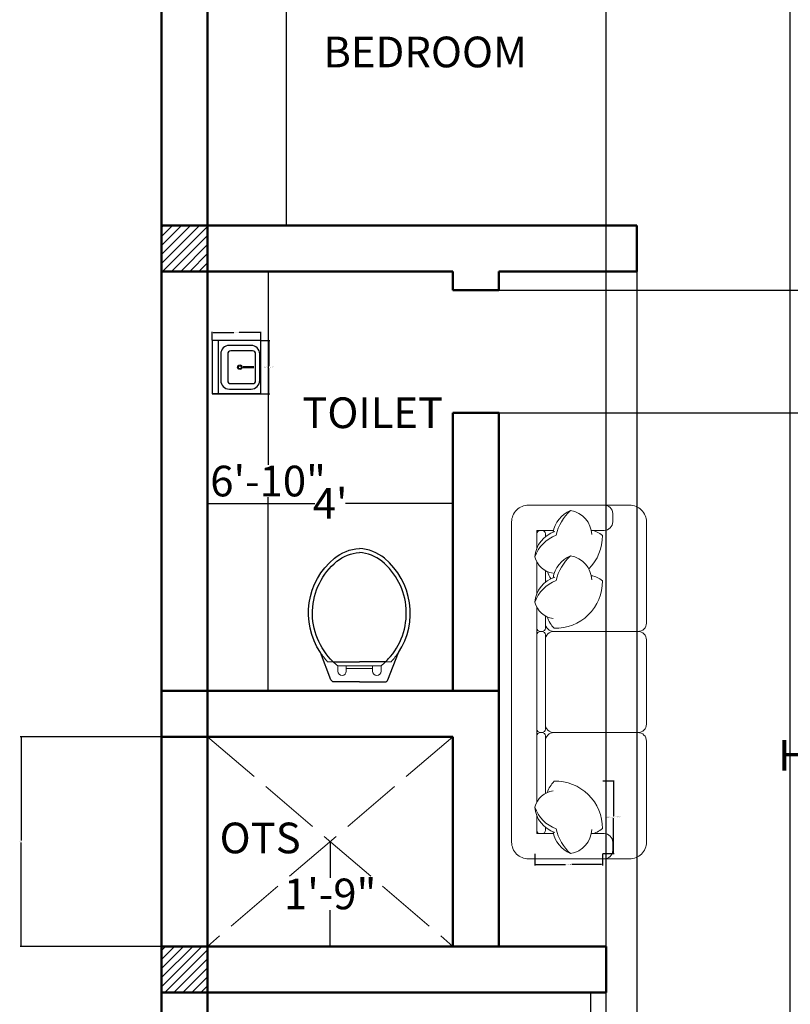
# Model space of a CAD drawing. Units: inches. Extents: x 0 to 281, y -535 to 46.
# Tile 3 of 22: x 0 to 150, y -275 to -82. Entities that reach past the tile are written whole.
import ezdxf

# ---------------------------------------------------------------- set-up
doc = ezdxf.new("R2010")
doc.units = ezdxf.units.IN
doc.header["$MEASUREMENT"] = 0
doc.linetypes.add('ACAD_ISO02W100', pattern=[15, 12, -3])
for name, color, linetype, lineweight in [('A-ANNO-DIMS', 2, 'Continuous', 18), ('A-AREA-IDEN', 7, 'Continuous', 25), ('A-COLS-PATT', 152, 'Continuous', 13), ('A-FLOR-FIXT', 9, 'Continuous', 25), ('A-FLOR-OPEN', 8, 'ACAD_ISO02W100', 13), ('A-FURN', 8, 'Continuous', 18), ('A-WALL', 7, 'Continuous', 50), ('WC-Detail_dwgmodels.com', 251, 'Continuous', 13), ('WC-Outline_dwgmodels.com', 250, 'Continuous', 25)]:
    doc.layers.add(name, color=color, linetype=linetype, lineweight=lineweight)
doc.styles.get("Standard").update_dxf_attribs({"font": 'arial.ttf'})
doc.dimstyles.get("Standard").update_dxf_attribs({"dimtxt": 0.18, "dimasz": 0.18, "dimexe": 0.18, "dimexo": 0.0625, "dimgap": 0.09, "dimtad": 0, "dimtih": 1, "dimtoh": 1, "dimdec": 0, "dimzin": 0, "dimdsep": 46, "dimlunit": 3, "dimtxsty": 'Standard', "dimcen": 0.09, "dimadec": 0, "dimazin": 0, "dimtfac": 1, "dimtdec": 0, "dimtofl": 0, "dimtmove": 0, "dimatfit": 3, "dimfxl": 1, "dimtolj": 1, "dimtzin": 0, "dimarcsym": 0})

# ---------------------------------------------------------------- blocks, each defined once
blk = doc.blocks.new('*D1')
at = {"layer": 'A-ANNO-DIMS', "color": 0, "lineweight": -2, "transparency": 16777216}
for p, q in [((51.94, 9.41), (51.94, -53.31)), ((52, 9.59), (52.12, 9.59)), ((51.94, -122.23), (51.94, -59.51)), ((52, -122.41), (52.12, -122.41))]:
    blk.add_line(p, q, dxfattribs=at)
at = {"layer": 'A-ANNO-DIMS', "color": 0, "transparency": 16777216}
for points in [[(51.91, 9.41), (51.97, 9.41), (51.94, 9.59)], [(51.91, -122.23), (51.97, -122.23), (51.94, -122.41)]]:
    blk.add_solid(points, dxfattribs=at)
at = {"layer": 'Defpoints', "color": 0, "transparency": 16777216}
for p in [(51.94, 9.59), (51.94, -122.41), (51.94, -122.41)]:
    blk.add_point(p, dxfattribs=at)
at = {"layer": 'A-ANNO-DIMS', "color": 0, "transparency": 16777216, "insert": (51.94, -56.41), "char_height": 6, "attachment_point": 5}
blk.add_mtext("\\A1;11'", dxfattribs=at)
blk = doc.blocks.new('*D5')
at = {"layer": 'A-ANNO-DIMS', "color": 0, "lineweight": -2, "transparency": 16777216}
for p, q in [((93.46, -158.99), (93.46, -158.87)), ((93.64, -159.05), (153.85, -159.05)), ((234.28, -159.05), (174.07, -159.05)), ((234.46, -158.99), (234.46, -158.87))]:
    blk.add_line(p, q, dxfattribs=at)
at = {"layer": 'A-ANNO-DIMS', "color": 0, "transparency": 16777216}
for points in [[(93.64, -159.02), (93.64, -159.08), (93.46, -159.05)], [(234.28, -159.02), (234.28, -159.08), (234.46, -159.05)]]:
    blk.add_solid(points, dxfattribs=at)
at = {"layer": 'Defpoints', "color": 0, "transparency": 16777216}
for p in [(93.46, -159.05), (234.46, -159.05), (234.46, -159.05)]:
    blk.add_point(p, dxfattribs=at)
at = {"layer": 'A-ANNO-DIMS', "color": 0, "transparency": 16777216, "insert": (163.96, -159.05), "char_height": 6, "attachment_point": 5}
blk.add_mtext('\\A1;11\'-9"', dxfattribs=at)
blk = doc.blocks.new('*D7')
at = {"layer": 'A-ANNO-DIMS', "color": 0, "lineweight": -2, "transparency": 16777216}
for p, q in [((48.25, -131.41), (48.14, -131.41)), ((48.32, -131.59), (48.32, -169.26)), ((48.32, -213.23), (48.32, -175.56)), ((48.38, -213.41), (48.5, -213.41))]:
    blk.add_line(p, q, dxfattribs=at)
at = {"layer": 'A-ANNO-DIMS', "color": 0, "transparency": 16777216}
for points in [[(48.29, -131.59), (48.35, -131.59), (48.32, -131.41)], [(48.29, -213.23), (48.35, -213.23), (48.32, -213.41)]]:
    blk.add_solid(points, dxfattribs=at)
at = {"layer": 'Defpoints', "color": 0, "transparency": 16777216}
for p in [(48.32, -131.41), (48.32, -213.41), (48.32, -213.41)]:
    blk.add_point(p, dxfattribs=at)
at = {"layer": 'A-ANNO-DIMS', "color": 0, "transparency": 16777216, "insert": (48.32, -172.41), "char_height": 6, "attachment_point": 5}
blk.add_mtext('\\A1;6\'-10"', dxfattribs=at)
blk = doc.blocks.new('*D8')
at = {"layer": 'A-ANNO-DIMS', "color": 0, "lineweight": -2, "transparency": 16777216}
for p, q in [((36.46, -176.98), (36.46, -176.61)), ((36.64, -176.79), (57.49, -176.79)), ((84.28, -176.79), (63.43, -176.79)), ((84.46, -176.98), (84.46, -176.61))]:
    blk.add_line(p, q, dxfattribs=at)
at = {"layer": 'A-ANNO-DIMS', "color": 0, "transparency": 16777216}
for points in [[(36.64, -176.76), (36.64, -176.82), (36.46, -176.79)], [(84.28, -176.76), (84.28, -176.82), (84.46, -176.79)]]:
    blk.add_solid(points, dxfattribs=at)
at = {"layer": 'Defpoints', "color": 0, "transparency": 16777216}
for p in [(36.46, -176.79), (36.46, -177.04), (84.46, -177.04)]:
    blk.add_point(p, dxfattribs=at)
at = {"layer": 'A-ANNO-DIMS', "color": 0, "transparency": 16777216, "insert": (60.46, -176.79), "char_height": 6, "attachment_point": 5}
blk.add_mtext("\\A1;4'", dxfattribs=at)
blk = doc.blocks.new('*D9')
at = {"layer": 'A-ANNO-DIMS', "color": 0, "lineweight": -2, "transparency": 16777216}
for p, q in [((114.4, -272.41), (111.21, -272.41)), ((111.39, -272.59), (111.39, -329.26)), ((111.39, -392.23), (111.39, -335.56)), ((114.4, -392.41), (111.21, -392.41))]:
    blk.add_line(p, q, dxfattribs=at)
at = {"layer": 'A-ANNO-DIMS', "color": 0, "transparency": 16777216}
for points in [[(111.36, -272.59), (111.42, -272.59), (111.39, -272.41)], [(111.36, -392.23), (111.42, -392.23), (111.39, -392.41)]]:
    blk.add_solid(points, dxfattribs=at)
at = {"layer": 'Defpoints', "color": 0, "transparency": 16777216}
for p in [(111.39, -272.41), (114.46, -272.41), (114.46, -392.41)]:
    blk.add_point(p, dxfattribs=at)
at = {"layer": 'A-ANNO-DIMS', "color": 0, "transparency": 16777216, "insert": (111.39, -332.41), "char_height": 6, "attachment_point": 5}
blk.add_mtext("\\A1;10'", dxfattribs=at)
blk = doc.blocks.new('М14 600х655')
for p, q in [((-655, 600), (-655, 0)), ((-655, 600), (-655, 0)), ((-655, 0), (-655, 600)), ((0, 600), (-655, 600)), ((0, 525), (-655, 525)), ((-165, 494), (-490, 494)), ((0, 0), (0, 600)), ((-596, 388), (-596, 121)), ((-528, 370), (-528, 103)), ((-165, 408), (-490, 408)), ((-127, 103), (-127, 370)), ((-59, 121), (-59, 388)), ((-334, 87), (-334, 220)), ((-321, 87), (-321, 220)), ((-655, 0), (-655, 0)), ((-655, 0), (-655, 0)), ((-655, 0), (0, 0)), ((-655, 0), (0, 0)), ((-490, 65), (-165, 65)), ((-490, 15), (-165, 15))]:
    blk.add_line(p, q)
for radius in [27.6, 19.3]:
    blk.add_circle((-327, 259), radius)
for centre, radius, start, end in [((-490, 388), 106, 90, 180), ((-165, 388), 106, 0, 90), ((-490, 370), 38.2, 90, 180), ((-165, 370), 38.2, 0, 90), ((-490, 121), 106, 180, 270), ((-165, 121), 106, 270, 0), ((-490, 103), 38.2, 180, 270), ((-165, 103), 38.2, 270, 0)]:
    blk.add_arc(centre, radius, start, end)
blk = doc.blocks.new('*D20')
at = {"layer": 'A-ANNO-DIMS', "color": 0, "lineweight": -2, "transparency": 16777216}
for p, q in [((60.46, -243.09), (60.46, -250.01)), ((60.52, -242.91), (60.64, -242.91)), ((60.46, -263.23), (60.46, -256.31)), ((60.52, -263.41), (60.64, -263.41))]:
    blk.add_line(p, q, dxfattribs=at)
at = {"layer": 'A-ANNO-DIMS', "color": 0, "transparency": 16777216}
for points in [[(60.43, -243.09), (60.49, -243.09), (60.46, -242.91)], [(60.43, -263.23), (60.49, -263.23), (60.46, -263.41)]]:
    blk.add_solid(points, dxfattribs=at)
at = {"layer": 'Defpoints', "color": 0, "transparency": 16777216}
for p in [(60.46, -242.91), (60.46, -263.41), (60.46, -263.41)]:
    blk.add_point(p, dxfattribs=at)
at = {"layer": 'A-ANNO-DIMS', "color": 0, "transparency": 16777216, "insert": (60.46, -253.16), "char_height": 6, "attachment_point": 5}
blk.add_mtext('\\A1;1\'-9"', dxfattribs=at)
blk = doc.blocks.new('SOFA-THROW-PILLOW')
for points in [[(11.04, 3.89, 0.165541), (13.21, 4.91, 0.425989), (3.78, 14.16, 0.121523), (2.47, 11.97, -7.115464)], [(3.93, 4.15, -0.306663), (0, 9.06, -0.30633), (3.59, 12.27, 0.872847)], [(6.98, 0, -0.14773), (4.15, 4.82, -0.213343), (0, 9.06, -0.178662)], [(11.14, 4.72, -0.356772), (6.98, 0, -0.249542), (3.56, 4.28, 9.61688)]]:
    blk.add_lwpolyline(points, format="xyb")
blk = doc.blocks.new('*D28')
at = {"layer": 'A-ANNO-DIMS', "color": 0, "lineweight": -2, "transparency": 16777216}
for p, q in [((113.79, -231.03), (116.04, -231.03)), ((115.86, -231.21), (115.86, -237.96)), ((115.86, -245.09), (115.86, -238.33)), ((113.79, -245.27), (116.04, -245.27))]:
    blk.add_line(p, q, dxfattribs=at)
at = {"layer": 'A-ANNO-DIMS', "color": 0, "transparency": 16777216}
for points in [[(115.83, -231.21), (115.89, -231.21), (115.86, -231.03)], [(115.83, -245.09), (115.89, -245.09), (115.86, -245.27)]]:
    blk.add_solid(points, dxfattribs=at)
at = {"layer": 'Defpoints', "color": 0, "transparency": 16777216}
for p in [(113.73, -231.03), (115.86, -231.03), (113.73, -245.27)]:
    blk.add_point(p, dxfattribs=at)
at = {"layer": 'A-ANNO-DIMS', "color": 0, "transparency": 16777216, "insert": (115.86, -238.15), "char_height": 0.18, "attachment_point": 5}
blk.add_mtext('\\A1;SOFA CUSHION 1\'-2" TYP.', dxfattribs=at)
blk = doc.blocks.new('*D29')
at = {"layer": 'A-ANNO-DIMS', "color": 0, "lineweight": -2, "transparency": 16777216}
for p, q in [((100.49, -245.33), (100.49, -247.58)), ((113.73, -245.33), (113.73, -247.58)), ((100.67, -247.4), (106.48, -247.4)), ((113.55, -247.4), (107.74, -247.4))]:
    blk.add_line(p, q, dxfattribs=at)
at = {"layer": 'A-ANNO-DIMS', "color": 0, "transparency": 16777216}
for points in [[(100.67, -247.37), (100.67, -247.43), (100.49, -247.4)], [(113.55, -247.37), (113.55, -247.43), (113.73, -247.4)]]:
    blk.add_solid(points, dxfattribs=at)
at = {"layer": 'Defpoints', "color": 0, "transparency": 16777216}
for p in [(100.49, -245.27), (113.73, -245.27), (113.73, -247.4)]:
    blk.add_point(p, dxfattribs=at)
at = {"layer": 'A-ANNO-DIMS', "color": 0, "transparency": 16777216, "insert": (107.11, -247.4), "char_height": 0.18, "attachment_point": 5}
blk.add_mtext('\\A1;1\'-1" TYP.', dxfattribs=at)
blk = doc.blocks.new('*D32')
at = {"layer": 'A-ANNO-DIMS', "color": 0, "lineweight": -2, "transparency": 16777216}
for p, q in [((46.98, -144.95), (48.67, -144.95)), ((48.49, -145.13), (48.49, -149.97)), ((48.49, -155.19), (48.49, -150.34)), ((46.98, -155.37), (48.67, -155.37))]:
    blk.add_line(p, q, dxfattribs=at)
at = {"layer": 'A-ANNO-DIMS', "color": 0, "transparency": 16777216}
for points in [[(48.46, -145.13), (48.52, -145.13), (48.49, -144.95)], [(48.46, -155.19), (48.52, -155.19), (48.49, -155.37)]]:
    blk.add_solid(points, dxfattribs=at)
at = {"layer": 'Defpoints', "color": 0, "transparency": 16777216}
for p in [(46.92, -144.95), (48.49, -144.95), (46.92, -155.37)]:
    blk.add_point(p, dxfattribs=at)
at = {"layer": 'A-ANNO-DIMS', "color": 0, "transparency": 16777216, "insert": (48.49, -150.16), "char_height": 0.18, "attachment_point": 5}
blk.add_mtext('\\A1;BASIN 0\'-10 1/2"', dxfattribs=at)
blk = doc.blocks.new('*D33')
at = {"layer": 'A-ANNO-DIMS', "color": 0, "lineweight": -2, "transparency": 16777216}
for p, q in [((37.37, -144.88), (37.37, -143.2)), ((37.55, -143.38), (41.61, -143.38)), ((46.74, -143.38), (42.69, -143.38)), ((46.92, -144.88), (46.92, -143.2))]:
    blk.add_line(p, q, dxfattribs=at)
at = {"layer": 'A-ANNO-DIMS', "color": 0, "transparency": 16777216}
for points in [[(37.55, -143.35), (37.55, -143.41), (37.37, -143.38)], [(46.74, -143.35), (46.74, -143.41), (46.92, -143.38)]]:
    blk.add_solid(points, dxfattribs=at)
at = {"layer": 'Defpoints', "color": 0, "transparency": 16777216}
for p in [(37.37, -143.38), (37.37, -144.95), (46.92, -144.95)]:
    blk.add_point(p, dxfattribs=at)
at = {"layer": 'A-ANNO-DIMS', "color": 0, "transparency": 16777216, "insert": (42.15, -143.38), "char_height": 0.18, "attachment_point": 5}
blk.add_mtext('\\A1;0\'-9 1/2"', dxfattribs=at)
blk = doc.blocks.new('*D41')
at = {"layer": 'A-ANNO-DIMS', "color": 0, "lineweight": -2, "transparency": 16777216}
for p, q in [((120.46, -131.47), (120.46, -535.04)), ((156.46, -131.47), (156.46, -535.04)), ((120.64, -534.86), (138.13, -534.86)), ((156.28, -534.86), (138.79, -534.86))]:
    blk.add_line(p, q, dxfattribs=at)
at = {"layer": 'A-ANNO-DIMS', "color": 0, "transparency": 16777216}
for points in [[(120.64, -534.83), (120.64, -534.89), (120.46, -534.86)], [(156.28, -534.83), (156.28, -534.89), (156.46, -534.86)]]:
    blk.add_solid(points, dxfattribs=at)
at = {"layer": 'Defpoints', "color": 0, "transparency": 16777216}
for p in [(120.46, -131.41), (156.46, -131.41), (156.46, -534.86)]:
    blk.add_point(p, dxfattribs=at)
at = {"layer": 'A-ANNO-DIMS', "color": 0, "transparency": 16777216, "insert": (138.46, -534.86), "char_height": 0.18, "attachment_point": 5}
blk.add_mtext('\\A1;3\'-0"', dxfattribs=at)
blk = doc.blocks.new('*D43')
at = {"layer": 'A-ANNO-DIMS', "color": 0, "lineweight": -2, "transparency": 16777216}
for p, q in [((93.52, -135.05), (271.09, -135.05)), ((270.91, -135.23), (270.91, -146.87)), ((270.91, -158.87), (270.91, -147.23)), ((93.52, -159.05), (271.09, -159.05))]:
    blk.add_line(p, q, dxfattribs=at)
at = {"layer": 'A-ANNO-DIMS', "color": 0, "transparency": 16777216}
for points in [[(270.88, -135.23), (270.94, -135.23), (270.91, -135.05)], [(270.88, -158.87), (270.94, -158.87), (270.91, -159.05)]]:
    blk.add_solid(points, dxfattribs=at)
at = {"layer": 'Defpoints', "color": 0, "transparency": 16777216}
for p in [(93.46, -135.05), (93.46, -159.05), (270.91, -159.05)]:
    blk.add_point(p, dxfattribs=at)
at = {"layer": 'A-ANNO-DIMS', "color": 0, "transparency": 16777216, "insert": (270.91, -147.05), "char_height": 0.18, "attachment_point": 5}
blk.add_mtext('\\A1;2\'-0"', dxfattribs=at)
blk = doc.blocks.new('*D44')
at = {"layer": 'A-ANNO-DIMS', "color": 0, "lineweight": -2, "transparency": 16777216}
for p, q in [((36.4, -222.41), (-0.17, -222.41)), ((0.01, -222.59), (0.01, -242.73)), ((0.01, -263.23), (0.01, -243.09)), ((36.4, -263.41), (-0.17, -263.41))]:
    blk.add_line(p, q, dxfattribs=at)
at = {"layer": 'A-ANNO-DIMS', "color": 0, "transparency": 16777216}
for points in [[(-0.02, -222.59), (0.04, -222.59), (0.01, -222.41)], [(-0.02, -263.23), (0.04, -263.23), (0.01, -263.41)]]:
    blk.add_solid(points, dxfattribs=at)
at = {"layer": 'Defpoints', "color": 0, "transparency": 16777216}
for p in [(36.46, -222.41), (0.01, -263.41), (36.46, -263.41)]:
    blk.add_point(p, dxfattribs=at)
at = {"layer": 'A-ANNO-DIMS', "color": 0, "transparency": 16777216, "insert": (0.01, -242.91), "char_height": 0.18, "attachment_point": 5}
blk.add_mtext('\\A1;3\'-5"', dxfattribs=at)
blk = doc.blocks.new('*D45')
at = {"layer": 'A-ANNO-DIMS', "color": 0, "lineweight": -2, "transparency": 16777216}
for p, q in [((114.46, -263.35), (114.46, 46.22)), ((150.46, -263.35), (150.46, 46.22)), ((114.64, 46.04), (132.13, 46.04)), ((150.28, 46.04), (132.79, 46.04))]:
    blk.add_line(p, q, dxfattribs=at)
at = {"layer": 'A-ANNO-DIMS', "color": 0, "transparency": 16777216}
for points in [[(114.64, 46.07), (114.64, 46.01), (114.46, 46.04)], [(150.28, 46.07), (150.28, 46.01), (150.46, 46.04)]]:
    blk.add_solid(points, dxfattribs=at)
at = {"layer": 'Defpoints', "color": 0, "transparency": 16777216}
for p in [(150.46, 46.04), (114.46, -263.41), (150.46, -263.41)]:
    blk.add_point(p, dxfattribs=at)
at = {"layer": 'A-ANNO-DIMS', "color": 0, "transparency": 16777216, "insert": (132.46, 46.04), "char_height": 0.18, "attachment_point": 5}
blk.add_mtext('\\A1;3\'-0"', dxfattribs=at)
blk = doc.blocks.new('*D47')
at = {"layer": 'A-ANNO-DIMS', "color": 0, "lineweight": -2, "transparency": 16777216}
for p, q in [((114.46, -392.35), (114.46, 46.22)), ((150.46, -392.35), (150.46, 46.22)), ((114.64, 46.04), (132.13, 46.04)), ((150.28, 46.04), (132.79, 46.04))]:
    blk.add_line(p, q, dxfattribs=at)
at = {"layer": 'A-ANNO-DIMS', "color": 0, "transparency": 16777216}
for points in [[(114.64, 46.07), (114.64, 46.01), (114.46, 46.04)], [(150.28, 46.07), (150.28, 46.01), (150.46, 46.04)]]:
    blk.add_solid(points, dxfattribs=at)
at = {"layer": 'Defpoints', "color": 0, "transparency": 16777216}
for p in [(150.46, 46.04), (114.46, -392.41), (150.46, -392.41)]:
    blk.add_point(p, dxfattribs=at)
at = {"layer": 'A-ANNO-DIMS', "color": 0, "transparency": 16777216, "insert": (132.46, 46.04), "char_height": 0.18, "attachment_point": 5}
blk.add_mtext('\\A1;3\'-0"', dxfattribs=at)

msp = doc.modelspace()

# ---------------------------------------------------------------- hatches: boundary and pattern name
at = {"layer": 'A-COLS-PATT'}
h = msp.add_hatch(dxfattribs=at)
h.set_pattern_fill('ANSI31', color=256, scale=10)
h.paths.add_polyline_path([(36.46, 18.59), (27.46, 18.59), (27.46, 9.59), (36.46, 9.59)])
h.paths.add_polyline_path([(165.46, 18.59), (156.46, 18.59), (156.46, 9.59), (165.46, 9.59)])
h.paths.add_polyline_path([(243.46, 18.59), (234.46, 18.59), (234.46, 9.59), (243.46, 9.59)])
h.paths.add_polyline_path([(243.46, -122.41), (234.46, -122.41), (234.46, -131.41), (243.46, -131.41)])
h.paths.add_polyline_path([(36.46, -122.41), (27.46, -122.41), (27.46, -131.41), (36.46, -131.41)])
h.paths.add_polyline_path([(36.46, -498.41), (27.46, -498.41), (27.46, -507.41), (36.46, -507.41)])
h.paths.add_polyline_path([(243.46, -498.41), (234.46, -498.41), (234.46, -507.41), (243.46, -507.41)])
h.paths.add_polyline_path([(159.46, -498.41), (150.46, -498.41), (150.46, -507.41), (159.46, -507.41)])
h.paths.add_polyline_path([(36.46, -392.41), (27.46, -392.41), (27.46, -401.41), (36.46, -401.41)])
h.paths.add_polyline_path([(159.46, -392.41), (150.46, -392.41), (150.46, -401.41), (159.46, -401.41)])
h.paths.add_polyline_path([(243.46, -392.41), (234.46, -392.41), (234.46, -401.41), (243.46, -401.41)])
h.paths.add_polyline_path([(36.46, -263.41), (27.46, -263.41), (27.46, -272.41), (36.46, -272.41)])
h.paths.add_polyline_path([(243.46, -263.41), (234.46, -263.41), (234.46, -272.41), (243.46, -272.41)])

# ---------------------------------------------------------------- linework, layer by layer
at = {"layer": 'A-FLOR-OPEN'}
for p, q in [((36.46, -222.41), (84.46, -263.41)), ((84.46, -222.41), (36.46, -263.41))]:
    msp.add_line(p, q, dxfattribs=at)
at = {"layer": 'A-FURN', "ltscale": 0.03}
msp.add_lwpolyline([(119.02, -246.31, 0.414214), (122.32, -243.02), (122.32, -223.25, 0.414214), (120.67, -221.6, 0.414214), (122.32, -219.95), (122.32, -203.48, 0.414214), (120.67, -201.83, 0.414214), (122.32, -200.18), (122.32, -180.41, 0.414214), (119.02, -177.12), (99.25, -177.12, 0.414214), (95.95, -180.41), (95.95, -243.02, 0.414214), (99.25, -246.31)], format="xyb", close=True, dxfattribs=at)
at = {"layer": 'A-FURN'}
for points in [[(111.53, -182.06), (114.08, -182.06, 0.414214), (115.73, -180.41), (115.73, -178.76, 0.414214), (114.08, -177.12)], [(107.47, -178.16, 0.14773), (104.64, -182.98, 0.213343), (100.49, -187.23, 0.178662)], [(111.63, -182.89, 0.356772), (107.47, -178.16, 0.249542), (104.05, -182.44, -9.61688)], [(104.42, -182.31, 0.306663), (100.49, -187.23, 0.30633), (104.07, -190.44, -0.872847)], [(100.9, -185.52), (100.9, -182.06), (104.14, -182.06, 0.414214)], [(102.55, -183.32), (102.55, -182.72, 0.414214), (101.89, -182.06), (101.56, -182.06, 0.414214), (100.9, -182.72)], [(100.9, -182.72), (100.9, -185.52, 0.414214)], [(111.52, -182.06, -0.165541), (113.7, -183.07, -0.200231), (111.05, -189.61, -0.121523)], [(100.9, -188.27), (100.9, -194.4, 0.414214)], [(102.55, -192.19), (102.55, -189.92, 0.414214)], [(103.61, -191.51, -0.071865), (102.96, -190.13, 7.115464)], [(100.9, -197.14), (100.9, -201.17, 0.414214), (101.56, -201.83), (101.89, -201.83, 0.414214), (102.55, -201.17), (102.55, -198.8, 0.414214)], [(102.55, -200.18, 0.414214), (104.19, -201.83), (120.67, -201.83, 0.414214)], [(102.55, -203.48, -0.414214), (104.19, -201.83)], [(102.55, -219.95, 0.414214), (104.19, -221.6)], [(100.9, -235.16), (100.9, -222.26, -0.414214), (101.56, -221.6), (101.89, -221.6, -0.414214), (102.55, -222.26), (102.55, -233.51, -0.414214)], [(102.55, -223.25, -0.414214), (104.19, -221.6), (120.67, -221.6, -0.414214)], [(100.9, -240.71), (100.9, -237.91, -0.414214)], [(102.55, -240.11), (102.55, -240.71, -0.414214), (101.89, -241.37), (101.56, -241.37, -0.414214), (100.9, -240.71)], [(114.08, -246.31, 0.414214), (115.73, -244.67), (115.73, -243.02, 0.414214), (114.08, -241.37), (111.53, -241.37)]]:
    msp.add_lwpolyline(points, format="xyb", dxfattribs=at)
for points in [[(100.9, -194.4), (100.9, -188.27)], [(100.9, -235.16), (100.9, -197.14)], [(104.14, -241.37), (100.9, -241.37), (100.9, -237.91)]]:
    msp.add_lwpolyline(points, dxfattribs=at)
msp.add_lwpolyline([(100.9, -202.49), (100.9, -220.94, 0.414214), (101.56, -221.6), (101.89, -221.6, 0.414214), (102.55, -220.94), (102.55, -202.49, 0.414214), (101.89, -201.83), (101.56, -201.83, 0.414214)], format="xyb", close=True, dxfattribs=at)
at = {"layer": 'A-WALL'}
for p, q in [((27.46, 18.59), (27.46, -507.41)), ((36.46, 18.59), (36.46, -507.41)), ((27.46, -122.41), (120.46, -122.41)), ((120.46, -131.41), (120.46, -122.41)), ((27.46, -131.41), (84.46, -131.41)), ((84.46, -131.41), (84.46, -135.05)), ((93.46, -131.41), (93.46, -135.05)), ((93.46, -131.41), (120.46, -131.41)), ((84.46, -135.05), (93.46, -135.05)), ((93.46, -159.05), (84.46, -159.05)), ((84.46, -159.05), (84.46, -213.41)), ((93.46, -159.05), (93.46, -263.41)), ((27.46, -213.41), (93.46, -213.41)), ((27.46, -222.41), (84.46, -222.41)), ((84.46, -222.41), (84.46, -263.41)), ((27.46, -263.41), (114.46, -263.41)), ((114.46, -272.41), (114.46, -263.41)), ((27.46, -272.41), (114.46, -272.41))]:
    msp.add_line(p, q, dxfattribs=at)
at = {"layer": 'WC-Detail_dwgmodels.com'}
for p, q in [((61.05, -207.74), (59.96, -207.74)), ((72.4, -207.74), (71.31, -207.74))]:
    msp.add_line(p, q, dxfattribs=at)
for points in [[(59.96, -207.74, -0.040937), (58.55, -205.95, -0.163732)], [(72.4, -207.74, 0.040937), (73.81, -205.95, 0.163732)], [(61.95, -208.53, -0.022712), (61.05, -207.74, -0.162618)], [(70.41, -208.53, 0.022712), (71.31, -207.74, 0.162618)], [(66.18, -208.53), (61.95, -208.53, -0.476108)], [(61.95, -208.53), (61.95, -209.62, 1), (63.61, -209.62), (63.61, -209.05)], [(66.18, -208.53), (70.41, -208.53, 0.022712)], [(70.41, -208.53), (70.41, -209.62, -1), (68.75, -209.62), (68.75, -209.05)]]:
    msp.add_lwpolyline(points, format="xyb", dxfattribs=at)
for points in [[(63.61, -209.05), (63.61, -208.53)], [(63.61, -209.05), (68.75, -209.05)], [(68.75, -209.05), (68.75, -208.53)]]:
    msp.add_lwpolyline(points, dxfattribs=at)
at = {"layer": 'WC-Outline_dwgmodels.com'}
for p in [(61.05, -207.74), (71.31, -207.74)]:
    msp.add_line(p, (66.18, -207.74), dxfattribs=at)
for points in [[(58.55, -205.95, -0.383919), (61.28, -187.51, -0.163732), (66.18, -185.63, -0.359733)], [(61.05, -207.74, -0.448546), (61.78, -188.11, -0.162618), (66.18, -186.41, -0.470877)], [(73.81, -205.95, 0.383919), (71.08, -187.51, 0.163732), (66.18, -185.63, 0.359733)], [(71.83, -207.21, 0.431639), (70.58, -188.11, 0.162618), (66.18, -186.41, 0.470877)], [(66.18, -211.68), (61.2, -211.68, -0.31031), (60.6, -211.27), (58.55, -205.95, -0.209071)], [(66.18, -211.68), (71.15, -211.68, 0.31031), (71.76, -211.27), (73.81, -205.95, 0.209071)], [(71.31, -207.74, 0.014165), (71.83, -207.21, 0.162618)]]:
    msp.add_lwpolyline(points, format="xyb", dxfattribs=at)

# ---------------------------------------------------------------- block references
at = {"layer": 'A-FLOR-FIXT', "xscale": 0.0159155461302873, "yscale": 0.0159155461302873, "zscale": 0.0159155461302873, "rotation": 90}
msp.add_blockref('М14 600х655', (46.92, -144.95), dxfattribs=at)
at = {"layer": 'A-FURN', "extrusion": (0, 0, -1), "zscale": -1, "rotation": 180}
msp.add_blockref('SOFA-THROW-PILLOW', (-100.49, -187.04), dxfattribs=at)
at = {"layer": 'A-FURN'}
msp.add_blockref('SOFA-THROW-PILLOW', (100.49, -245.27), dxfattribs=at)

# ---------------------------------------------------------------- texts
at = {"layer": 'A-AREA-IDEN', "char_height": 6, "attachment_point": 1}
for s, insert in [('BEDROOM', (59.14, -85.5)), ('TOILET', (55.01, -156.06)), ('HALL+DINING', (148.07, -223.05)), ('OTS', (38.84, -239.21))]:
    msp.add_mtext(s, dxfattribs=dict(at, insert=insert))

# ---------------------------------------------------------------- dimensions: what is measured, and where the dimension line sits
at = {"layer": 'A-ANNO-DIMS'}
for base, p1, p2, override, picture, middle in [((150.46, 46.04), (114.46, -263.41), (150.46, -263.41), {"dimdec": 1, "dimlfac": 1, "dimrnd": 0, "dimzin": 1, "dimdsep": 46, "dimlunit": 4, "dimfrac": 2}, '*D45', (132.46, 46.04)), ((150.46, 46.04), (114.46, -392.41), (150.46, -392.41), {"dimdec": 1, "dimlfac": 1, "dimrnd": 0, "dimzin": 1, "dimdsep": 46, "dimlunit": 4, "dimfrac": 2}, '*D47', (132.46, 46.04)), ((156.46, -534.86), (120.46, -131.41), (156.46, -131.41), {"dimdec": 1, "dimlfac": 1, "dimrnd": 0, "dimzin": 1, "dimdsep": 46, "dimlunit": 4, "dimfrac": 2}, '*D41', (138.46, -534.86)), ((234.46, -159.05), (93.46, -159.05), (234.46, -159.05), {"dimtxt": 6, "dimclrd": 0, "dimclre": 0, "dimclrt": 0}, '*D5', (163.96, -159.05)), ((36.46, -176.79), (84.46, -177.04), (36.46, -177.04), {"dimtxt": 6, "dimclrd": 0, "dimclre": 0, "dimclrt": 0}, '*D8', (60.46, -176.79))]:
    dim = msp.add_linear_dim(base=base, p1=p1, p2=p2, dimstyle='Standard', override=override, dxfattribs=at)
    dim.commit()
    dim.dimension.update_dxf_attribs({"geometry": picture, "text_midpoint": middle})
for base, p1, p2, angle, override, picture, middle in [((51.94, -122.41), (51.94, 9.59), (51.94, -122.41), 90, {"dimtxt": 6, "dimclrd": 0, "dimclre": 0, "dimclrt": 0}, '*D1', (51.94, -56.41)), ((48.32, -213.41), (48.32, -131.41), (48.32, -213.41), 90, {"dimtxt": 6, "dimclrd": 0, "dimclre": 0, "dimclrt": 0}, '*D7', (48.32, -172.41)), ((270.91, -159.05), (93.46, -135.05), (93.46, -159.05), 90, {"dimdec": 1, "dimlfac": 1, "dimrnd": 0, "dimzin": 1, "dimdsep": 46, "dimlunit": 4, "dimfrac": 2}, '*D43', (270.91, -147.05)), ((37.3729, -143.3816), (46.9222, -144.9453), (37.3729, -144.9453), 180, {"dimdec": 1, "dimlfac": 1, "dimrnd": 0, "dimzin": 1, "dimdsep": 46, "dimlunit": 4, "dimfrac": 2}, '*D33', (42.1475, -143.3816)), ((0.01, -263.41), (36.46, -222.41), (36.46, -263.41), 90, {"dimdec": 1, "dimlfac": 1, "dimrnd": 0, "dimzin": 1, "dimdsep": 46, "dimlunit": 4, "dimfrac": 2}, '*D44', (0.01, -242.91)), ((60.45886315, -263.41051508), (60.45886315, -242.91051508), (60.45886315, -263.41051508), 90, {"dimtxt": 6, "dimclrd": 0, "dimclre": 0, "dimclrt": 0}, '*D20', (60.45886315, -253.16051508)), ((111.39, -272.41), (114.46, -392.41), (114.46, -272.41), 90, {"dimtxt": 6, "dimclrd": 0, "dimclre": 0, "dimclrt": 0}, '*D9', (111.39, -332.41))]:
    dim = msp.add_linear_dim(base=base, p1=p1, p2=p2, angle=angle, dimstyle='Standard', override=override, dxfattribs=at)
    dim.commit()
    dim.dimension.update_dxf_attribs({"geometry": picture, "text_midpoint": middle})
for base, p1, p2, text, picture, middle in [((48.49, -144.95), (46.92, -155.37), (46.92, -144.95), 'BASIN <>', '*D32', (48.49, -150.16)), ((115.86, -231.03), (113.73, -245.27), (113.73, -231.03), 'SOFA CUSHION <> TYP.', '*D28', (115.86, -238.15))]:
    dim = msp.add_linear_dim(base=base, p1=p1, p2=p2, angle=90, text=text, dimstyle='Standard', override={"dimdec": 1, "dimlfac": 1, "dimrnd": 0, "dimzin": 1, "dimdsep": 46, "dimlunit": 4, "dimfrac": 2}, dxfattribs=at)
    dim.commit()
    dim.dimension.update_dxf_attribs({"geometry": picture, "text_midpoint": middle})
dim = msp.add_linear_dim(base=(113.73, -247.4), p1=(100.49, -245.27), p2=(113.73, -245.27), text='<> TYP.', dimstyle='Standard', override={"dimdec": 1, "dimlfac": 1, "dimrnd": 0, "dimzin": 1, "dimdsep": 46, "dimlunit": 4, "dimfrac": 2}, dxfattribs=at)
dim.commit()
dim.dimension.update_dxf_attribs({"geometry": '*D29', "text_midpoint": (107.11, -247.4)})

doc.saveas('drawing.dxf')
